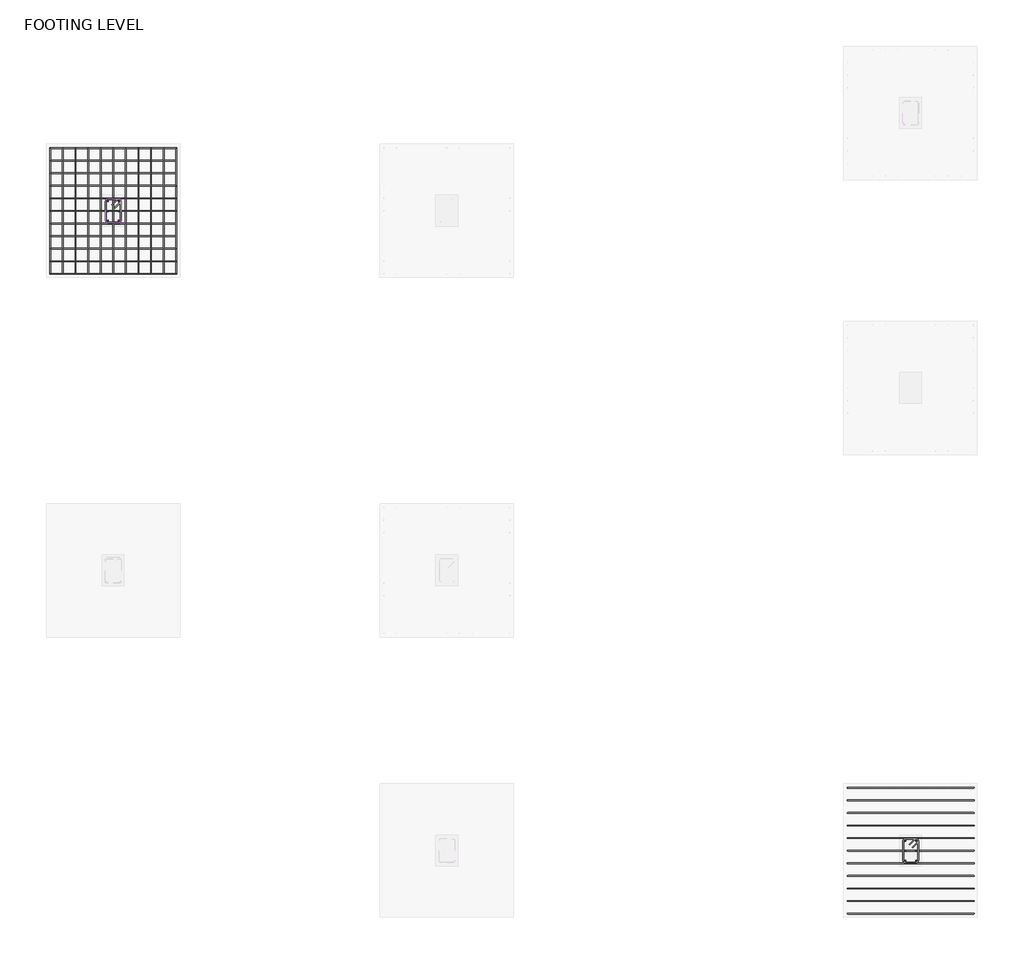
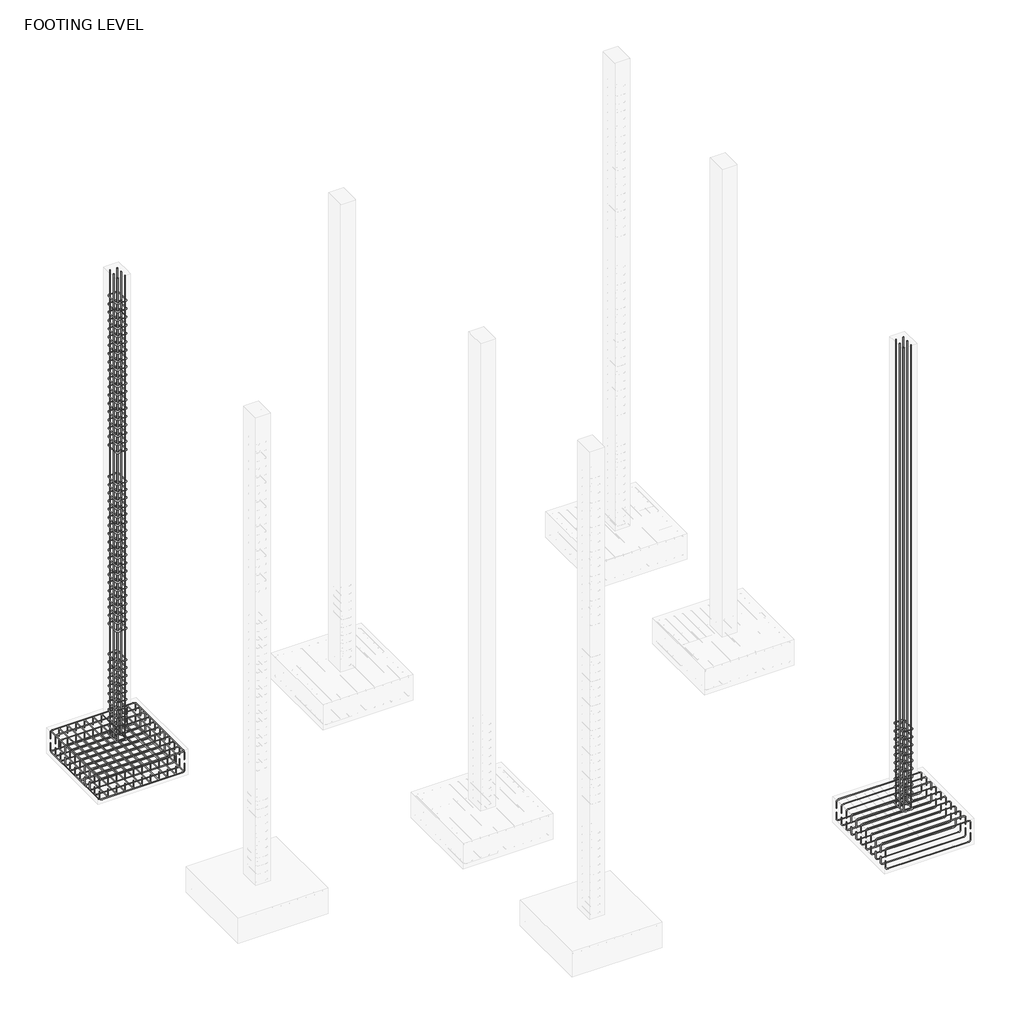
# One storey, part 4 of 9: 22 reinforcing bars.
"""IFC4 building model written with IfcOpenShell, lengths in millimetres."""

from ifc_helpers import new_model, si_unit, point, frame, origin, place, context, project, spatial, polyline, circle_curve, trimmed, segment, composite_curve, source, transform, mapped, element, save
from ifc_brep_helpers import swept_disk

model = new_model("IFC4")

# Units and contexts
model_context = context("Model", 3, world=origin())
ifc_project = project(units=[si_unit("LENGTHUNIT", "METRE", prefix="MILLI")], contexts=[model_context])

# Site, building, storey
site = spatial("IfcSite", under=ifc_project)
building = spatial("IfcBuilding", under=site)
storey = spatial("IfcBuildingStorey", under=building, Name="FOOTING LEVEL", Elevation=-1981.2)

# Reinforcing bars
placement = place(None, origin())
reinforcing_bar_shape = source(origin(), model_context, "Body", "SolidModel", [
    swept_disk(composite_curve([segment(polyline([(-3975.4566189, -3042.2841598, -2171.7), (-3975.4566189, -3042.2841598, -2057.4)]), True, "CONTINUOUS"), segment(trimmed(circle_curve(frame((-3942.1191189, -3042.2841598, -2057.4), z_axis=(0.0, 1.0, 0.0), x_axis=(-33.33750000000009, 0.0, 0.0)), 33.3375), [point((-3975.4566189, -3042.2841598, -2057.4))], [point((-3942.1191189, -3042.2841598, -2024.0625))], True, "CARTESIAN"), True, "CONTINUOUS"), segment(polyline([(-3942.1191189, -3042.2841598, -2024.0625), (-2570.5191189, -3042.2841598, -2024.0625)]), True, "CONTINUOUS"), segment(trimmed(circle_curve(frame((-2570.5191189, -3042.2841598, -2057.4), z_axis=(0.0, 1.0, 0.0), x_axis=(0.0, 0.0, 33.33750000000009)), 33.3375), [point((-2570.5191189, -3042.2841598, -2024.0625))], [point((-2537.1816189, -3042.2841598, -2057.4))], True, "CARTESIAN"), True, "CONTINUOUS"), segment(polyline([(-2537.1816189, -3042.2841598, -2057.4), (-2537.1816189, -3042.2841598, -2171.7)]), True, "CONTINUOUS")], self_intersect=False), 4.7625),
])
element("IfcReinforcingBar", 1, at=placement, inside=storey, context=model_context, shape_type="MappedRepresentation", body=[
    mapped(reinforcing_bar_shape, transform((0.0, 0.0, 0.0), x_axis=(1.0, 0.0, 0.0), y_axis=(0.0, 1.0, 0.0), z_axis=(0.0, 0.0, 1.0))),
    mapped(reinforcing_bar_shape, transform((0.0, -143.8275, 0.0), x_axis=(1.0, 0.0, 0.0), y_axis=(0.0, 1.0, 0.0), z_axis=(0.0, 0.0, 1.0))),
    mapped(reinforcing_bar_shape, transform((0.0, -287.655, 0.0), x_axis=(1.0, 0.0, 0.0), y_axis=(0.0, 1.0, 0.0), z_axis=(0.0, 0.0, 1.0))),
    mapped(reinforcing_bar_shape, transform((0.0, -431.4825, 0.0), x_axis=(1.0, 0.0, 0.0), y_axis=(0.0, 1.0, 0.0), z_axis=(0.0, 0.0, 1.0))),
    mapped(reinforcing_bar_shape, transform((0.0, -575.31, 0.0), x_axis=(1.0, 0.0, 0.0), y_axis=(0.0, 1.0, 0.0), z_axis=(0.0, 0.0, 1.0))),
    mapped(reinforcing_bar_shape, transform((0.0, -719.1375, 0.0), x_axis=(1.0, 0.0, 0.0), y_axis=(0.0, 1.0, 0.0), z_axis=(0.0, 0.0, 1.0))),
    mapped(reinforcing_bar_shape, transform((0.0, -862.965, 0.0), x_axis=(1.0, 0.0, 0.0), y_axis=(0.0, 1.0, 0.0), z_axis=(0.0, 0.0, 1.0))),
    mapped(reinforcing_bar_shape, transform((0.0, -1006.7925, 0.0), x_axis=(1.0, 0.0, 0.0), y_axis=(0.0, 1.0, 0.0), z_axis=(0.0, 0.0, 1.0))),
    mapped(reinforcing_bar_shape, transform((0.0, -1150.62, 0.0), x_axis=(1.0, 0.0, 0.0), y_axis=(0.0, 1.0, 0.0), z_axis=(0.0, 0.0, 1.0))),
    mapped(reinforcing_bar_shape, transform((0.0, -1294.4475, 0.0), x_axis=(1.0, 0.0, 0.0), y_axis=(0.0, 1.0, 0.0), z_axis=(0.0, 0.0, 1.0))),
    mapped(reinforcing_bar_shape, transform((0.0, -1438.275, 0.0), x_axis=(1.0, 0.0, 0.0), y_axis=(0.0, 1.0, 0.0), z_axis=(0.0, 0.0, 1.0))),
])
reinforcing_bar_2_shape = source(origin(), model_context, "Body", "SolidModel", [
    swept_disk(composite_curve([segment(polyline([(-3975.4566189, -4480.5591598, -2247.9), (-3975.4566189, -4480.5591598, -2362.2)]), True, "CONTINUOUS"), segment(trimmed(circle_curve(frame((-3942.1191189, -4480.5591598, -2362.2), z_axis=(0.0, -1.0, 0.0), x_axis=(-33.33750000000009, 0.0, 0.0)), 33.3375), [point((-3975.4566189, -4480.5591598, -2362.2))], [point((-3942.1191189, -4480.5591598, -2395.5375))], True, "CARTESIAN"), True, "CONTINUOUS"), segment(polyline([(-3942.1191189, -4480.5591598, -2395.5375), (-2570.5191189, -4480.5591598, -2395.5375)]), True, "CONTINUOUS"), segment(trimmed(circle_curve(frame((-2570.5191189, -4480.5591598, -2362.2), z_axis=(0.0, -1.0, 0.0), x_axis=(0.0, 0.0, -33.33750000000009)), 33.3375), [point((-2570.5191189, -4480.5591598, -2395.5375))], [point((-2537.1816189, -4480.5591598, -2362.2))], True, "CARTESIAN"), True, "CONTINUOUS"), segment(polyline([(-2537.1816189, -4480.5591598, -2362.2), (-2537.1816189, -4480.5591598, -2247.9)]), True, "CONTINUOUS")], self_intersect=False), 4.7625),
])
element("IfcReinforcingBar", 2, at=placement, inside=storey, context=model_context, shape_type="MappedRepresentation", body=[
    mapped(reinforcing_bar_2_shape, transform((0.0, 0.0, 0.0), x_axis=(1.0, 0.0, 0.0), y_axis=(0.0, 1.0, 0.0), z_axis=(0.0, 0.0, 1.0))),
    mapped(reinforcing_bar_2_shape, transform((0.0, 143.8275, 0.0), x_axis=(1.0, 0.0, 0.0), y_axis=(0.0, 1.0, 0.0), z_axis=(0.0, 0.0, 1.0))),
    mapped(reinforcing_bar_2_shape, transform((0.0, 287.655, 0.0), x_axis=(1.0, 0.0, 0.0), y_axis=(0.0, 1.0, 0.0), z_axis=(0.0, 0.0, 1.0))),
    mapped(reinforcing_bar_2_shape, transform((0.0, 431.4825, 0.0), x_axis=(1.0, 0.0, 0.0), y_axis=(0.0, 1.0, 0.0), z_axis=(0.0, 0.0, 1.0))),
    mapped(reinforcing_bar_2_shape, transform((0.0, 575.31, 0.0), x_axis=(1.0, 0.0, 0.0), y_axis=(0.0, 1.0, 0.0), z_axis=(0.0, 0.0, 1.0))),
    mapped(reinforcing_bar_2_shape, transform((0.0, 719.1375, 0.0), x_axis=(1.0, 0.0, 0.0), y_axis=(0.0, 1.0, 0.0), z_axis=(0.0, 0.0, 1.0))),
    mapped(reinforcing_bar_2_shape, transform((0.0, 862.965, 0.0), x_axis=(1.0, 0.0, 0.0), y_axis=(0.0, 1.0, 0.0), z_axis=(0.0, 0.0, 1.0))),
    mapped(reinforcing_bar_2_shape, transform((0.0, 1006.7925, 0.0), x_axis=(1.0, 0.0, 0.0), y_axis=(0.0, 1.0, 0.0), z_axis=(0.0, 0.0, 1.0))),
    mapped(reinforcing_bar_2_shape, transform((0.0, 1150.62, 0.0), x_axis=(1.0, 0.0, 0.0), y_axis=(0.0, 1.0, 0.0), z_axis=(0.0, 0.0, 1.0))),
    mapped(reinforcing_bar_2_shape, transform((0.0, 1294.4475, 0.0), x_axis=(1.0, 0.0, 0.0), y_axis=(0.0, 1.0, 0.0), z_axis=(0.0, 0.0, 1.0))),
    mapped(reinforcing_bar_2_shape, transform((0.0, 1438.275, 0.0), x_axis=(1.0, 0.0, 0.0), y_axis=(0.0, 1.0, 0.0), z_axis=(0.0, 0.0, 1.0))),
])
reinforcing_bar_3_shape = source(origin(), model_context, "Body", "SolidModel", [
    swept_disk(composite_curve([segment(polyline([(-11642.9458659, 4266.5658402, -2171.7), (-11642.9458659, 4266.5658402, -2057.4)]), True, "CONTINUOUS"), segment(trimmed(circle_curve(frame((-11642.9458659, 4233.2283402, -2057.4), z_axis=(1.0, 0.0, 0.0), x_axis=(0.0, 33.337499999999636, 0.0)), 33.3375), [point((-11642.9458659, 4266.5658402, -2057.4))], [point((-11642.9458659, 4233.2283402, -2024.0625))], True, "CARTESIAN"), True, "CONTINUOUS"), segment(polyline([(-11642.9458659, 4233.2283402, -2024.0625), (-11642.9458659, 2861.6283402, -2024.0625)]), True, "CONTINUOUS"), segment(trimmed(circle_curve(frame((-11642.9458659, 2861.6283402, -2057.4), z_axis=(1.0, 0.0, 0.0), x_axis=(0.0, 0.0, 33.33750000000009)), 33.3375), [point((-11642.9458659, 2861.6283402, -2024.0625))], [point((-11642.9458659, 2828.2908402, -2057.4))], True, "CARTESIAN"), True, "CONTINUOUS"), segment(polyline([(-11642.9458659, 2828.2908402, -2057.4), (-11642.9458659, 2828.2908402, -2171.7)]), True, "CONTINUOUS")], self_intersect=False), 4.7625),
])
element("IfcReinforcingBar", 3, at=placement, inside=storey, context=model_context, shape_type="MappedRepresentation", body=[
    mapped(reinforcing_bar_3_shape, transform((0.0, 0.0, 0.0), x_axis=(1.0, 0.0, 0.0), y_axis=(0.0, 1.0, 0.0), z_axis=(0.0, 0.0, 1.0))),
    mapped(reinforcing_bar_3_shape, transform((-143.8275, 0.0, 0.0), x_axis=(1.0, 0.0, 0.0), y_axis=(0.0, 1.0, 0.0), z_axis=(0.0, 0.0, 1.0))),
    mapped(reinforcing_bar_3_shape, transform((-287.655, 0.0, 0.0), x_axis=(1.0, 0.0, 0.0), y_axis=(0.0, 1.0, 0.0), z_axis=(0.0, 0.0, 1.0))),
    mapped(reinforcing_bar_3_shape, transform((-431.4825, 0.0, 0.0), x_axis=(1.0, 0.0, 0.0), y_axis=(0.0, 1.0, 0.0), z_axis=(0.0, 0.0, 1.0))),
    mapped(reinforcing_bar_3_shape, transform((-575.31, 0.0, 0.0), x_axis=(1.0, 0.0, 0.0), y_axis=(0.0, 1.0, 0.0), z_axis=(0.0, 0.0, 1.0))),
    mapped(reinforcing_bar_3_shape, transform((-719.1375, 0.0, 0.0), x_axis=(1.0, 0.0, 0.0), y_axis=(0.0, 1.0, 0.0), z_axis=(0.0, 0.0, 1.0))),
    mapped(reinforcing_bar_3_shape, transform((-862.965, 0.0, 0.0), x_axis=(1.0, 0.0, 0.0), y_axis=(0.0, 1.0, 0.0), z_axis=(0.0, 0.0, 1.0))),
    mapped(reinforcing_bar_3_shape, transform((-1006.7925, 0.0, 0.0), x_axis=(1.0, 0.0, 0.0), y_axis=(0.0, 1.0, 0.0), z_axis=(0.0, 0.0, 1.0))),
    mapped(reinforcing_bar_3_shape, transform((-1150.62, 0.0, 0.0), x_axis=(1.0, 0.0, 0.0), y_axis=(0.0, 1.0, 0.0), z_axis=(0.0, 0.0, 1.0))),
    mapped(reinforcing_bar_3_shape, transform((-1294.4475, 0.0, 0.0), x_axis=(1.0, 0.0, 0.0), y_axis=(0.0, 1.0, 0.0), z_axis=(0.0, 0.0, 1.0))),
    mapped(reinforcing_bar_3_shape, transform((-1438.275, 0.0, 0.0), x_axis=(1.0, 0.0, 0.0), y_axis=(0.0, 1.0, 0.0), z_axis=(0.0, 0.0, 1.0))),
])
reinforcing_bar_4_shape = source(origin(), model_context, "Body", "SolidModel", [
    swept_disk(composite_curve([segment(polyline([(-11642.9458659, 2828.2908402, -2247.9), (-11642.9458659, 2828.2908402, -2362.2)]), True, "CONTINUOUS"), segment(trimmed(circle_curve(frame((-11642.9458659, 2861.6283402, -2362.2), z_axis=(1.0, 0.0, 0.0), x_axis=(0.0, -33.33750000000009, 0.0)), 33.3375), [point((-11642.9458659, 2828.2908402, -2362.2))], [point((-11642.9458659, 2861.6283402, -2395.5375))], True, "CARTESIAN"), True, "CONTINUOUS"), segment(polyline([(-11642.9458659, 2861.6283402, -2395.5375), (-11642.9458659, 4233.2283402, -2395.5375)]), True, "CONTINUOUS"), segment(trimmed(circle_curve(frame((-11642.9458659, 4233.2283402, -2362.2), z_axis=(1.0, 0.0, 0.0), x_axis=(0.0, 0.0, -33.33750000000009)), 33.3375), [point((-11642.9458659, 4233.2283402, -2395.5375))], [point((-11642.9458659, 4266.5658402, -2362.2))], True, "CARTESIAN"), True, "CONTINUOUS"), segment(polyline([(-11642.9458659, 4266.5658402, -2362.2), (-11642.9458659, 4266.5658402, -2247.9)]), True, "CONTINUOUS")], self_intersect=False), 4.7625),
])
element("IfcReinforcingBar", 4, at=placement, inside=storey, context=model_context, shape_type="MappedRepresentation", body=[
    mapped(reinforcing_bar_4_shape, transform((0.0, 0.0, 0.0), x_axis=(1.0, 0.0, 0.0), y_axis=(0.0, 1.0, 0.0), z_axis=(0.0, 0.0, 1.0))),
    mapped(reinforcing_bar_4_shape, transform((-143.8275, 0.0, 0.0), x_axis=(1.0, 0.0, 0.0), y_axis=(0.0, 1.0, 0.0), z_axis=(0.0, 0.0, 1.0))),
    mapped(reinforcing_bar_4_shape, transform((-287.655, 0.0, 0.0), x_axis=(1.0, 0.0, 0.0), y_axis=(0.0, 1.0, 0.0), z_axis=(0.0, 0.0, 1.0))),
    mapped(reinforcing_bar_4_shape, transform((-431.4825, 0.0, 0.0), x_axis=(1.0, 0.0, 0.0), y_axis=(0.0, 1.0, 0.0), z_axis=(0.0, 0.0, 1.0))),
    mapped(reinforcing_bar_4_shape, transform((-575.31, 0.0, 0.0), x_axis=(1.0, 0.0, 0.0), y_axis=(0.0, 1.0, 0.0), z_axis=(0.0, 0.0, 1.0))),
    mapped(reinforcing_bar_4_shape, transform((-719.1375, 0.0, 0.0), x_axis=(1.0, 0.0, 0.0), y_axis=(0.0, 1.0, 0.0), z_axis=(0.0, 0.0, 1.0))),
    mapped(reinforcing_bar_4_shape, transform((-862.965, 0.0, 0.0), x_axis=(1.0, 0.0, 0.0), y_axis=(0.0, 1.0, 0.0), z_axis=(0.0, 0.0, 1.0))),
    mapped(reinforcing_bar_4_shape, transform((-1006.7925, 0.0, 0.0), x_axis=(1.0, 0.0, 0.0), y_axis=(0.0, 1.0, 0.0), z_axis=(0.0, 0.0, 1.0))),
    mapped(reinforcing_bar_4_shape, transform((-1150.62, 0.0, 0.0), x_axis=(1.0, 0.0, 0.0), y_axis=(0.0, 1.0, 0.0), z_axis=(0.0, 0.0, 1.0))),
    mapped(reinforcing_bar_4_shape, transform((-1294.4475, 0.0, 0.0), x_axis=(1.0, 0.0, 0.0), y_axis=(0.0, 1.0, 0.0), z_axis=(0.0, 0.0, 1.0))),
    mapped(reinforcing_bar_4_shape, transform((-1438.275, 0.0, 0.0), x_axis=(1.0, 0.0, 0.0), y_axis=(0.0, 1.0, 0.0), z_axis=(0.0, 0.0, 1.0))),
])
reinforcing_bar_5_shape = source(origin(), model_context, "Body", "SolidModel", [
    swept_disk(composite_curve([segment(polyline([(-13081.2208659, 4266.5658402, -2171.7), (-13081.2208659, 4266.5658402, -2057.4)]), True, "CONTINUOUS"), segment(trimmed(circle_curve(frame((-13047.8833659, 4266.5658402, -2057.4), z_axis=(0.0, 1.0, 0.0), x_axis=(-33.337500000001455, 0.0, 0.0)), 33.3375), [point((-13081.2208659, 4266.5658402, -2057.4))], [point((-13047.8833659, 4266.5658402, -2024.0625))], True, "CARTESIAN"), True, "CONTINUOUS"), segment(polyline([(-13047.8833659, 4266.5658402, -2024.0625), (-11676.2833659, 4266.5658402, -2024.0625)]), True, "CONTINUOUS"), segment(trimmed(circle_curve(frame((-11676.2833659, 4266.5658402, -2057.4), z_axis=(0.0, 1.0, 0.0), x_axis=(0.0, 0.0, 33.33750000000009)), 33.3375), [point((-11676.2833659, 4266.5658402, -2024.0625))], [point((-11642.9458659, 4266.5658402, -2057.4))], True, "CARTESIAN"), True, "CONTINUOUS"), segment(polyline([(-11642.9458659, 4266.5658402, -2057.4), (-11642.9458659, 4266.5658402, -2171.7)]), True, "CONTINUOUS")], self_intersect=False), 4.7625),
])
element("IfcReinforcingBar", 5, at=placement, inside=storey, context=model_context, shape_type="MappedRepresentation", body=[
    mapped(reinforcing_bar_5_shape, transform((0.0, 0.0, 0.0), x_axis=(1.0, 0.0, 0.0), y_axis=(0.0, 1.0, 0.0), z_axis=(0.0, 0.0, 1.0))),
    mapped(reinforcing_bar_5_shape, transform((0.0, -143.8275, 0.0), x_axis=(1.0, 0.0, 0.0), y_axis=(0.0, 1.0, 0.0), z_axis=(0.0, 0.0, 1.0))),
    mapped(reinforcing_bar_5_shape, transform((0.0, -287.655, 0.0), x_axis=(1.0, 0.0, 0.0), y_axis=(0.0, 1.0, 0.0), z_axis=(0.0, 0.0, 1.0))),
    mapped(reinforcing_bar_5_shape, transform((0.0, -431.4825, 0.0), x_axis=(1.0, 0.0, 0.0), y_axis=(0.0, 1.0, 0.0), z_axis=(0.0, 0.0, 1.0))),
    mapped(reinforcing_bar_5_shape, transform((0.0, -575.31, 0.0), x_axis=(1.0, 0.0, 0.0), y_axis=(0.0, 1.0, 0.0), z_axis=(0.0, 0.0, 1.0))),
    mapped(reinforcing_bar_5_shape, transform((0.0, -719.1375, 0.0), x_axis=(1.0, 0.0, 0.0), y_axis=(0.0, 1.0, 0.0), z_axis=(0.0, 0.0, 1.0))),
    mapped(reinforcing_bar_5_shape, transform((0.0, -862.965, 0.0), x_axis=(1.0, 0.0, 0.0), y_axis=(0.0, 1.0, 0.0), z_axis=(0.0, 0.0, 1.0))),
    mapped(reinforcing_bar_5_shape, transform((0.0, -1006.7925, 0.0), x_axis=(1.0, 0.0, 0.0), y_axis=(0.0, 1.0, 0.0), z_axis=(0.0, 0.0, 1.0))),
    mapped(reinforcing_bar_5_shape, transform((0.0, -1150.62, 0.0), x_axis=(1.0, 0.0, 0.0), y_axis=(0.0, 1.0, 0.0), z_axis=(0.0, 0.0, 1.0))),
    mapped(reinforcing_bar_5_shape, transform((0.0, -1294.4475, 0.0), x_axis=(1.0, 0.0, 0.0), y_axis=(0.0, 1.0, 0.0), z_axis=(0.0, 0.0, 1.0))),
    mapped(reinforcing_bar_5_shape, transform((0.0, -1438.275, 0.0), x_axis=(1.0, 0.0, 0.0), y_axis=(0.0, 1.0, 0.0), z_axis=(0.0, 0.0, 1.0))),
])
reinforcing_bar_6_shape = source(origin(), model_context, "Body", "SolidModel", [
    swept_disk(composite_curve([segment(polyline([(-13081.2208659, 2828.2908402, -2247.9), (-13081.2208659, 2828.2908402, -2362.2)]), True, "CONTINUOUS"), segment(trimmed(circle_curve(frame((-13047.8833659, 2828.2908402, -2362.2), z_axis=(0.0, -1.0, 0.0), x_axis=(-33.337500000001455, 0.0, 0.0)), 33.3375), [point((-13081.2208659, 2828.2908402, -2362.2))], [point((-13047.8833659, 2828.2908402, -2395.5375))], True, "CARTESIAN"), True, "CONTINUOUS"), segment(polyline([(-13047.8833659, 2828.2908402, -2395.5375), (-11676.2833659, 2828.2908402, -2395.5375)]), True, "CONTINUOUS"), segment(trimmed(circle_curve(frame((-11676.2833659, 2828.2908402, -2362.2), z_axis=(0.0, -1.0, 0.0), x_axis=(0.0, 0.0, -33.33750000000009)), 33.3375), [point((-11676.2833659, 2828.2908402, -2395.5375))], [point((-11642.9458659, 2828.2908402, -2362.2))], True, "CARTESIAN"), True, "CONTINUOUS"), segment(polyline([(-11642.9458659, 2828.2908402, -2362.2), (-11642.9458659, 2828.2908402, -2247.9)]), True, "CONTINUOUS")], self_intersect=False), 4.7625),
])
element("IfcReinforcingBar", 6, at=placement, inside=storey, context=model_context, shape_type="MappedRepresentation", body=[
    mapped(reinforcing_bar_6_shape, transform((0.0, 0.0, 0.0), x_axis=(1.0, 0.0, 0.0), y_axis=(0.0, 1.0, 0.0), z_axis=(0.0, 0.0, 1.0))),
    mapped(reinforcing_bar_6_shape, transform((0.0, 143.8275, 0.0), x_axis=(1.0, 0.0, 0.0), y_axis=(0.0, 1.0, 0.0), z_axis=(0.0, 0.0, 1.0))),
    mapped(reinforcing_bar_6_shape, transform((0.0, 287.655, 0.0), x_axis=(1.0, 0.0, 0.0), y_axis=(0.0, 1.0, 0.0), z_axis=(0.0, 0.0, 1.0))),
    mapped(reinforcing_bar_6_shape, transform((0.0, 431.4825, 0.0), x_axis=(1.0, 0.0, 0.0), y_axis=(0.0, 1.0, 0.0), z_axis=(0.0, 0.0, 1.0))),
    mapped(reinforcing_bar_6_shape, transform((0.0, 575.31, 0.0), x_axis=(1.0, 0.0, 0.0), y_axis=(0.0, 1.0, 0.0), z_axis=(0.0, 0.0, 1.0))),
    mapped(reinforcing_bar_6_shape, transform((0.0, 719.1375, 0.0), x_axis=(1.0, 0.0, 0.0), y_axis=(0.0, 1.0, 0.0), z_axis=(0.0, 0.0, 1.0))),
    mapped(reinforcing_bar_6_shape, transform((0.0, 862.965, 0.0), x_axis=(1.0, 0.0, 0.0), y_axis=(0.0, 1.0, 0.0), z_axis=(0.0, 0.0, 1.0))),
    mapped(reinforcing_bar_6_shape, transform((0.0, 1006.7925, 0.0), x_axis=(1.0, 0.0, 0.0), y_axis=(0.0, 1.0, 0.0), z_axis=(0.0, 0.0, 1.0))),
    mapped(reinforcing_bar_6_shape, transform((0.0, 1150.62, 0.0), x_axis=(1.0, 0.0, 0.0), y_axis=(0.0, 1.0, 0.0), z_axis=(0.0, 0.0, 1.0))),
    mapped(reinforcing_bar_6_shape, transform((0.0, 1294.4475, 0.0), x_axis=(1.0, 0.0, 0.0), y_axis=(0.0, 1.0, 0.0), z_axis=(0.0, 0.0, 1.0))),
    mapped(reinforcing_bar_6_shape, transform((0.0, 1438.275, 0.0), x_axis=(1.0, 0.0, 0.0), y_axis=(0.0, 1.0, 0.0), z_axis=(0.0, 0.0, 1.0))),
])
reinforcing_bar_7_shape = source(origin(), model_context, "Body", "SolidModel", [
    swept_disk(composite_curve([segment(polyline([(-12341.7845827, 3584.8511629, -1938.3375), (-12284.9203857, 3641.71536, -1938.3375)]), True, "CONTINUOUS"), segment(trimmed(circle_curve(frame((-12301.7583659, 3658.5533402, -1938.3375), z_axis=(0.0, 0.0, 1.0), x_axis=(16.837980199999947, -16.837980199999947, 0.0)), 23.8125), [point((-12284.9203857, 3641.71536, -1938.3375))], [point((-12301.7583659, 3682.3658402, -1938.3375))], True, "CARTESIAN"), True, "CONTINUOUS"), segment(polyline([(-12301.7583659, 3682.3658402, -1938.3375), (-12422.4083659, 3682.3658402, -1938.3375)]), True, "CONTINUOUS"), segment(trimmed(circle_curve(frame((-12422.4083659, 3658.5533402, -1938.3375), z_axis=(0.0, 0.0, 1.0), x_axis=(0.0, 23.8125, 0.0)), 23.8125), [point((-12422.4083659, 3682.3658402, -1938.3375))], [point((-12446.2208659, 3658.5533402, -1938.3375))], True, "CARTESIAN"), True, "CONTINUOUS"), segment(polyline([(-12446.2208659, 3658.5533402, -1938.3375), (-12446.2208659, 3436.3033402, -1938.3375)]), True, "CONTINUOUS"), segment(trimmed(circle_curve(frame((-12422.4464219, 3436.3033402, -1939.6832232), z_axis=(0.056513312022656255, 0.0, 0.9984018457335854), x_axis=(-23.774444000000585, 0.0, 1.3457231999998385)), 23.8125), [point((-12446.2208659, 3436.3033402, -1938.3375))], [point((-12422.4464219, 3412.4908402, -1939.6832232))], True, "CARTESIAN"), True, "CONTINUOUS"), segment(polyline([(-12422.4464219, 3412.4908402, -1939.6832232), (-12301.7203098, 3412.4908402, -1946.5167768)]), True, "CONTINUOUS"), segment(trimmed(circle_curve(frame((-12301.7203098, 3436.3033402, -1946.5167768), z_axis=(0.056513312022656255, 0.0, 0.9984018457335854), x_axis=(0.0, -23.8125, 0.0)), 23.8125), [point((-12301.7203098, 3412.4908402, -1946.5167768))], [point((-12277.9458659, 3436.3033402, -1947.8625))], True, "CARTESIAN"), True, "CONTINUOUS"), segment(polyline([(-12277.9458659, 3436.3033402, -1947.8625), (-12277.9458659, 3658.5533402, -1947.8625)]), True, "CONTINUOUS"), segment(trimmed(circle_curve(frame((-12301.7583659, 3658.5533402, -1947.8625), z_axis=(0.0, 0.0, 1.0), x_axis=(23.8125, 0.0, 0.0)), 23.8125), [point((-12277.9458659, 3658.5533402, -1947.8625))], [point((-12318.5963461, 3675.3913204, -1947.8625))], True, "CARTESIAN"), True, "CONTINUOUS"), segment(polyline([(-12318.5963461, 3675.3913204, -1947.8625), (-12375.4605432, 3618.5271233, -1947.8625)]), True, "CONTINUOUS")], self_intersect=False), 4.7625),
])
element("IfcReinforcingBar", 7, at=placement, inside=storey, context=model_context, shape_type="MappedRepresentation", body=[
    mapped(reinforcing_bar_7_shape, transform((0.0, 0.0, 0.0), x_axis=(1.0, 0.0, 0.0), y_axis=(0.0, 1.0, 0.0), z_axis=(0.0, 0.0, 1.0))),
    mapped(reinforcing_bar_7_shape, transform((0.0, 0.0, 142.5866456), x_axis=(1.0, 0.0, 0.0), y_axis=(0.0, 1.0, 0.0), z_axis=(0.0, 0.0, 1.0))),
    mapped(reinforcing_bar_7_shape, transform((0.0, 0.0, 285.1732912), x_axis=(1.0, 0.0, 0.0), y_axis=(0.0, 1.0, 0.0), z_axis=(0.0, 0.0, 1.0))),
    mapped(reinforcing_bar_7_shape, transform((0.0, 0.0, 427.7599369), x_axis=(1.0, 0.0, 0.0), y_axis=(0.0, 1.0, 0.0), z_axis=(0.0, 0.0, 1.0))),
    mapped(reinforcing_bar_7_shape, transform((0.0, 0.0, 570.3465825), x_axis=(1.0, 0.0, 0.0), y_axis=(0.0, 1.0, 0.0), z_axis=(0.0, 0.0, 1.0))),
    mapped(reinforcing_bar_7_shape, transform((0.0, 0.0, 712.9332281), x_axis=(1.0, 0.0, 0.0), y_axis=(0.0, 1.0, 0.0), z_axis=(0.0, 0.0, 1.0))),
    mapped(reinforcing_bar_7_shape, transform((0.0, 0.0, 855.5198737), x_axis=(1.0, 0.0, 0.0), y_axis=(0.0, 1.0, 0.0), z_axis=(0.0, 0.0, 1.0))),
    mapped(reinforcing_bar_7_shape, transform((0.0, 0.0, 998.1065193), x_axis=(1.0, 0.0, 0.0), y_axis=(0.0, 1.0, 0.0), z_axis=(0.0, 0.0, 1.0))),
    mapped(reinforcing_bar_7_shape, transform((0.0, 0.0, 1140.6931649), x_axis=(1.0, 0.0, 0.0), y_axis=(0.0, 1.0, 0.0), z_axis=(0.0, 0.0, 1.0))),
    mapped(reinforcing_bar_7_shape, transform((0.0, 0.0, 1283.2798106), x_axis=(1.0, 0.0, 0.0), y_axis=(0.0, 1.0, 0.0), z_axis=(0.0, 0.0, 1.0))),
    mapped(reinforcing_bar_7_shape, transform((0.0, 0.0, 1425.8664562), x_axis=(1.0, 0.0, 0.0), y_axis=(0.0, 1.0, 0.0), z_axis=(0.0, 0.0, 1.0))),
])
element("IfcReinforcingBar", 8, at=placement, inside=storey, context=model_context, shape_type="SolidModel", body=[
    swept_disk(composite_curve([segment(polyline([(-12300.2784581, 3433.9470011, -1943.1), (-12300.2784581, 3433.9470011, 6362.7)]), True, "CONTINUOUS")], self_intersect=False), 6.35),
])
element("IfcReinforcingBar", 9, at=placement, inside=storey, context=model_context, shape_type="SolidModel", body=[
    swept_disk(composite_curve([segment(polyline([(-12423.8882737, 3433.9470011, -1943.1), (-12423.8882737, 3433.9470011, 6362.7)]), True, "CONTINUOUS")], self_intersect=False), 6.35),
])
element("IfcReinforcingBar", 10, at=placement, inside=storey, context=model_context, shape_type="SolidModel", body=[
    swept_disk(composite_curve([segment(polyline([(-12300.2784581, 3660.9096793, -1943.1), (-12300.2784581, 3660.9096793, 6362.7)]), True, "CONTINUOUS")], self_intersect=False), 6.35),
])
element("IfcReinforcingBar", 11, at=placement, inside=storey, context=model_context, shape_type="SolidModel", body=[
    swept_disk(composite_curve([segment(polyline([(-12423.8882737, 3660.9096793, -1943.1), (-12423.8882737, 3660.9096793, 6362.7)]), True, "CONTINUOUS")], self_intersect=False), 6.35),
])
element("IfcReinforcingBar", 12, at=placement, inside=storey, context=model_context, shape_type="SolidModel", body=[
    swept_disk(composite_curve([segment(polyline([(-12300.2784581, 3546.6096793, -1943.1), (-12300.2784581, 3546.6096793, 6362.7)]), True, "CONTINUOUS")], self_intersect=False), 6.35),
])
element("IfcReinforcingBar", 13, at=placement, inside=storey, context=model_context, shape_type="SolidModel", body=[
    swept_disk(composite_curve([segment(polyline([(-12423.8882737, 3546.6096793, -1943.1), (-12423.8882737, 3546.6096793, 6362.7)]), True, "CONTINUOUS")], self_intersect=False), 6.35),
])
reinforcing_bar_8_shape = source(origin(), model_context, "Body", "SolidModel", [
    swept_disk(composite_curve([segment(polyline([(-3236.0203358, -3723.9988371, -1938.3375), (-3179.1561387, -3667.13464, -1938.3375)]), True, "CONTINUOUS"), segment(trimmed(circle_curve(frame((-3195.9941189, -3650.2966598, -1938.3375), z_axis=(0.0, 0.0, 1.0), x_axis=(16.837980199999947, -16.837980200000402, 0.0)), 23.8125), [point((-3179.1561387, -3667.13464, -1938.3375))], [point((-3195.9941189, -3626.4841598, -1938.3375))], True, "CARTESIAN"), True, "CONTINUOUS"), segment(polyline([(-3195.9941189, -3626.4841598, -1938.3375), (-3316.6441189, -3626.4841598, -1938.3375)]), True, "CONTINUOUS"), segment(trimmed(circle_curve(frame((-3316.6441189, -3650.2966598, -1938.3375), z_axis=(0.0, 0.0, 1.0), x_axis=(0.0, 23.8125, 0.0)), 23.8125), [point((-3316.6441189, -3626.4841598, -1938.3375))], [point((-3340.4566189, -3650.2966598, -1938.3375))], True, "CARTESIAN"), True, "CONTINUOUS"), segment(polyline([(-3340.4566189, -3650.2966598, -1938.3375), (-3340.4566189, -3872.5466598, -1938.3375)]), True, "CONTINUOUS"), segment(trimmed(circle_curve(frame((-3316.682175, -3872.5466598, -1939.6832232), z_axis=(0.056513312022656255, 0.0, 0.9984018457335854), x_axis=(-23.77444390000028, 0.0, 1.3457231999998385)), 23.8125), [point((-3340.4566189, -3872.5466598, -1938.3375))], [point((-3316.682175, -3896.3591598, -1939.6832232))], True, "CARTESIAN"), True, "CONTINUOUS"), segment(polyline([(-3316.682175, -3896.3591598, -1939.6832232), (-3195.9560629, -3896.3591598, -1946.5167768)]), True, "CONTINUOUS"), segment(trimmed(circle_curve(frame((-3195.9560629, -3872.5466598, -1946.5167768), z_axis=(0.056513312022656255, 0.0, 0.9984018457335854), x_axis=(0.0, -23.8125, 0.0)), 23.8125), [point((-3195.9560629, -3896.3591598, -1946.5167768))], [point((-3172.1816189, -3872.5466598, -1947.8625))], True, "CARTESIAN"), True, "CONTINUOUS"), segment(polyline([(-3172.1816189, -3872.5466598, -1947.8625), (-3172.1816189, -3650.2966598, -1947.8625)]), True, "CONTINUOUS"), segment(trimmed(circle_curve(frame((-3195.9941189, -3650.2966598, -1947.8625), z_axis=(0.0, 0.0, 1.0), x_axis=(23.8125, 0.0, 0.0)), 23.8125), [point((-3172.1816189, -3650.2966598, -1947.8625))], [point((-3212.8320991, -3633.4586796, -1947.8625))], True, "CARTESIAN"), True, "CONTINUOUS"), segment(polyline([(-3212.8320991, -3633.4586796, -1947.8625), (-3269.6962962, -3690.3228767, -1947.8625)]), True, "CONTINUOUS")], self_intersect=False), 4.7625),
])
element("IfcReinforcingBar", 14, at=placement, inside=storey, context=model_context, shape_type="MappedRepresentation", body=[
    mapped(reinforcing_bar_8_shape, transform((0.0, 0.0, 0.0), x_axis=(1.0, 0.0, 0.0), y_axis=(0.0, 1.0, 0.0), z_axis=(0.0, 0.0, 1.0))),
    mapped(reinforcing_bar_8_shape, transform((0.0, 0.0, 142.9363281), x_axis=(1.0, 0.0, 0.0), y_axis=(0.0, 1.0, 0.0), z_axis=(0.0, 0.0, 1.0))),
    mapped(reinforcing_bar_8_shape, transform((0.0, 0.0, 285.8726562), x_axis=(1.0, 0.0, 0.0), y_axis=(0.0, 1.0, 0.0), z_axis=(0.0, 0.0, 1.0))),
    mapped(reinforcing_bar_8_shape, transform((0.0, 0.0, 428.8089844), x_axis=(1.0, 0.0, 0.0), y_axis=(0.0, 1.0, 0.0), z_axis=(0.0, 0.0, 1.0))),
    mapped(reinforcing_bar_8_shape, transform((0.0, 0.0, 571.7453125), x_axis=(1.0, 0.0, 0.0), y_axis=(0.0, 1.0, 0.0), z_axis=(0.0, 0.0, 1.0))),
    mapped(reinforcing_bar_8_shape, transform((0.0, 0.0, 714.6816406), x_axis=(1.0, 0.0, 0.0), y_axis=(0.0, 1.0, 0.0), z_axis=(0.0, 0.0, 1.0))),
    mapped(reinforcing_bar_8_shape, transform((0.0, 0.0, 857.6179687), x_axis=(1.0, 0.0, 0.0), y_axis=(0.0, 1.0, 0.0), z_axis=(0.0, 0.0, 1.0))),
    mapped(reinforcing_bar_8_shape, transform((0.0, 0.0, 1000.5542969), x_axis=(1.0, 0.0, 0.0), y_axis=(0.0, 1.0, 0.0), z_axis=(0.0, 0.0, 1.0))),
    mapped(reinforcing_bar_8_shape, transform((0.0, 0.0, 1143.490625), x_axis=(1.0, 0.0, 0.0), y_axis=(0.0, 1.0, 0.0), z_axis=(0.0, 0.0, 1.0))),
    mapped(reinforcing_bar_8_shape, transform((0.0, 0.0, 1286.4269531), x_axis=(1.0, 0.0, 0.0), y_axis=(0.0, 1.0, 0.0), z_axis=(0.0, 0.0, 1.0))),
    mapped(reinforcing_bar_8_shape, transform((0.0, 0.0, 1429.3632812), x_axis=(1.0, 0.0, 0.0), y_axis=(0.0, 1.0, 0.0), z_axis=(0.0, 0.0, 1.0))),
])
element("IfcReinforcingBar", 15, at=placement, inside=storey, context=model_context, shape_type="SolidModel", body=[
    swept_disk(composite_curve([segment(polyline([(-3194.5142111, -3874.9029989, -1943.1), (-3194.5142111, -3874.9029989, 6362.7)]), True, "CONTINUOUS")], self_intersect=False), 6.35),
])
element("IfcReinforcingBar", 16, at=placement, inside=storey, context=model_context, shape_type="SolidModel", body=[
    swept_disk(composite_curve([segment(polyline([(-3318.1240267, -3874.9029989, -1943.1), (-3318.1240267, -3874.9029989, 6362.7)]), True, "CONTINUOUS")], self_intersect=False), 6.35),
])
element("IfcReinforcingBar", 17, at=placement, inside=storey, context=model_context, shape_type="SolidModel", body=[
    swept_disk(composite_curve([segment(polyline([(-3194.5142111, -3647.9403207, -1943.1), (-3194.5142111, -3647.9403207, 6362.7)]), True, "CONTINUOUS")], self_intersect=False), 6.35),
])
element("IfcReinforcingBar", 18, at=placement, inside=storey, context=model_context, shape_type="SolidModel", body=[
    swept_disk(composite_curve([segment(polyline([(-3318.1240267, -3647.9403207, -1943.1), (-3318.1240267, -3647.9403207, 6362.7)]), True, "CONTINUOUS")], self_intersect=False), 6.35),
])
element("IfcReinforcingBar", 19, at=placement, inside=storey, context=model_context, shape_type="SolidModel", body=[
    swept_disk(composite_curve([segment(polyline([(-3194.5142111, -3762.2403207, -1943.1), (-3194.5142111, -3762.2403207, 6362.7)]), True, "CONTINUOUS")], self_intersect=False), 6.35),
])
element("IfcReinforcingBar", 20, at=placement, inside=storey, context=model_context, shape_type="SolidModel", body=[
    swept_disk(composite_curve([segment(polyline([(-3318.1240267, -3762.2403207, -1943.1), (-3318.1240267, -3762.2403207, 6362.7)]), True, "CONTINUOUS")], self_intersect=False), 6.35),
])
reinforcing_bar_9_shape = source(origin(), model_context, "Body", "SolidModel", [
    swept_disk(composite_curve([segment(polyline([(-12382.3821491, 3510.0055175, 42.8625), (-12439.2463461, 3453.1413204, 42.8625)]), True, "CONTINUOUS"), segment(trimmed(circle_curve(frame((-12422.4083659, 3436.3033402, 42.8625), z_axis=(0.0, 0.0, 1.0), x_axis=(-16.837980199999947, 16.837980199999947, 0.0)), 23.8125), [point((-12439.2463461, 3453.1413204, 42.8625))], [point((-12422.4083659, 3412.4908402, 42.8625))], True, "CARTESIAN"), True, "CONTINUOUS"), segment(polyline([(-12422.4083659, 3412.4908402, 42.8625), (-12301.7583659, 3412.4908402, 42.8625)]), True, "CONTINUOUS"), segment(trimmed(circle_curve(frame((-12301.7583659, 3436.3033402, 42.8625), z_axis=(0.0, 0.0, 1.0), x_axis=(0.0, -23.8125, 0.0)), 23.8125), [point((-12301.7583659, 3412.4908402, 42.8625))], [point((-12277.9458659, 3436.3033402, 42.8625))], True, "CARTESIAN"), True, "CONTINUOUS"), segment(polyline([(-12277.9458659, 3436.3033402, 42.8625), (-12277.9458659, 3658.5533402, 42.8625)]), True, "CONTINUOUS"), segment(trimmed(circle_curve(frame((-12301.7203098, 3658.5533402, 41.5167768), z_axis=(-0.056513312022656255, 0.0, 0.9984018457335854), x_axis=(23.774443900001643, 0.0, 1.3457231999999948)), 23.8125), [point((-12277.9458659, 3658.5533402, 42.8625))], [point((-12301.7203098, 3682.3658402, 41.5167768))], True, "CARTESIAN"), True, "CONTINUOUS"), segment(polyline([(-12301.7203098, 3682.3658402, 41.5167768), (-12422.4464219, 3682.3658402, 34.6832232)]), True, "CONTINUOUS"), segment(trimmed(circle_curve(frame((-12422.4464219, 3658.5533402, 34.6832232), z_axis=(-0.056513312022656255, 0.0, 0.9984018457335854), x_axis=(0.0, 23.8125, 0.0)), 23.8125), [point((-12422.4464219, 3682.3658402, 34.6832232))], [point((-12446.2208659, 3658.5533402, 33.3375))], True, "CARTESIAN"), True, "CONTINUOUS"), segment(polyline([(-12446.2208659, 3658.5533402, 33.3375), (-12446.2208659, 3436.3033402, 33.3375)]), True, "CONTINUOUS"), segment(trimmed(circle_curve(frame((-12422.4083659, 3436.3033402, 33.3375), z_axis=(0.0, 0.0, 1.0), x_axis=(-23.8125, 0.0, 0.0)), 23.8125), [point((-12446.2208659, 3436.3033402, 33.3375))], [point((-12405.5703857, 3419.46536, 33.3375))], True, "CARTESIAN"), True, "CONTINUOUS"), segment(polyline([(-12405.5703857, 3419.46536, 33.3375), (-12348.7061886, 3476.329557, 33.3375)]), True, "CONTINUOUS")], self_intersect=False), 4.7625),
])
element("IfcReinforcingBar", 21, at=placement, inside=storey, context=model_context, shape_type="MappedRepresentation", body=[
    mapped(reinforcing_bar_9_shape, transform((0.0, 0.0, 0.0), x_axis=(1.0, 0.0, 0.0), y_axis=(0.0, 1.0, 0.0), z_axis=(0.0, 0.0, 1.0))),
    mapped(reinforcing_bar_9_shape, transform((0.0, 0.0, 146.2204368), x_axis=(1.0, 0.0, 0.0), y_axis=(0.0, 1.0, 0.0), z_axis=(0.0, 0.0, 1.0))),
    mapped(reinforcing_bar_9_shape, transform((0.0, 0.0, 292.4408736), x_axis=(1.0, 0.0, 0.0), y_axis=(0.0, 1.0, 0.0), z_axis=(0.0, 0.0, 1.0))),
    mapped(reinforcing_bar_9_shape, transform((0.0, 0.0, 438.6613104), x_axis=(1.0, 0.0, 0.0), y_axis=(0.0, 1.0, 0.0), z_axis=(0.0, 0.0, 1.0))),
    mapped(reinforcing_bar_9_shape, transform((0.0, 0.0, 584.8817472), x_axis=(1.0, 0.0, 0.0), y_axis=(0.0, 1.0, 0.0), z_axis=(0.0, 0.0, 1.0))),
    mapped(reinforcing_bar_9_shape, transform((0.0, 0.0, 731.102184), x_axis=(1.0, 0.0, 0.0), y_axis=(0.0, 1.0, 0.0), z_axis=(0.0, 0.0, 1.0))),
    mapped(reinforcing_bar_9_shape, transform((0.0, 0.0, 877.3226208), x_axis=(1.0, 0.0, 0.0), y_axis=(0.0, 1.0, 0.0), z_axis=(0.0, 0.0, 1.0))),
    mapped(reinforcing_bar_9_shape, transform((0.0, 0.0, 1023.5430576), x_axis=(1.0, 0.0, 0.0), y_axis=(0.0, 1.0, 0.0), z_axis=(0.0, 0.0, 1.0))),
    mapped(reinforcing_bar_9_shape, transform((0.0, 0.0, 1169.7634944), x_axis=(1.0, 0.0, 0.0), y_axis=(0.0, 1.0, 0.0), z_axis=(0.0, 0.0, 1.0))),
    mapped(reinforcing_bar_9_shape, transform((0.0, 0.0, 1315.9839312), x_axis=(1.0, 0.0, 0.0), y_axis=(0.0, 1.0, 0.0), z_axis=(0.0, 0.0, 1.0))),
    mapped(reinforcing_bar_9_shape, transform((0.0, 0.0, 1462.2043681), x_axis=(1.0, 0.0, 0.0), y_axis=(0.0, 1.0, 0.0), z_axis=(0.0, 0.0, 1.0))),
    mapped(reinforcing_bar_9_shape, transform((0.0, 0.0, 1608.4248049), x_axis=(1.0, 0.0, 0.0), y_axis=(0.0, 1.0, 0.0), z_axis=(0.0, 0.0, 1.0))),
    mapped(reinforcing_bar_9_shape, transform((0.0, 0.0, 1754.6452417), x_axis=(1.0, 0.0, 0.0), y_axis=(0.0, 1.0, 0.0), z_axis=(0.0, 0.0, 1.0))),
    mapped(reinforcing_bar_9_shape, transform((0.0, 0.0, 1900.8656785), x_axis=(1.0, 0.0, 0.0), y_axis=(0.0, 1.0, 0.0), z_axis=(0.0, 0.0, 1.0))),
    mapped(reinforcing_bar_9_shape, transform((0.0, 0.0, 2047.0861153), x_axis=(1.0, 0.0, 0.0), y_axis=(0.0, 1.0, 0.0), z_axis=(0.0, 0.0, 1.0))),
    mapped(reinforcing_bar_9_shape, transform((0.0, 0.0, 2193.3065521), x_axis=(1.0, 0.0, 0.0), y_axis=(0.0, 1.0, 0.0), z_axis=(0.0, 0.0, 1.0))),
    mapped(reinforcing_bar_9_shape, transform((0.0, 0.0, 2339.5269889), x_axis=(1.0, 0.0, 0.0), y_axis=(0.0, 1.0, 0.0), z_axis=(0.0, 0.0, 1.0))),
    mapped(reinforcing_bar_9_shape, transform((0.0, 0.0, 2485.7474257), x_axis=(1.0, 0.0, 0.0), y_axis=(0.0, 1.0, 0.0), z_axis=(0.0, 0.0, 1.0))),
    mapped(reinforcing_bar_9_shape, transform((0.0, 0.0, 2631.9678625), x_axis=(1.0, 0.0, 0.0), y_axis=(0.0, 1.0, 0.0), z_axis=(0.0, 0.0, 1.0))),
])
reinforcing_bar_10_shape = source(origin(), model_context, "Body", "SolidModel", [
    swept_disk(composite_curve([segment(polyline([(-12382.3821491, 3510.0055175, 3243.2625), (-12439.2463461, 3453.1413204, 3243.2625)]), True, "CONTINUOUS"), segment(trimmed(circle_curve(frame((-12422.4083659, 3436.3033402, 3243.2625), z_axis=(0.0, 0.0, 1.0), x_axis=(-16.837980199999947, 16.837980199999947, 0.0)), 23.8125), [point((-12439.2463461, 3453.1413204, 3243.2625))], [point((-12422.4083659, 3412.4908402, 3243.2625))], True, "CARTESIAN"), True, "CONTINUOUS"), segment(polyline([(-12422.4083659, 3412.4908402, 3243.2625), (-12301.7583659, 3412.4908402, 3243.2625)]), True, "CONTINUOUS"), segment(trimmed(circle_curve(frame((-12301.7583659, 3436.3033402, 3243.2625), z_axis=(0.0, 0.0, 1.0), x_axis=(0.0, -23.8125, 0.0)), 23.8125), [point((-12301.7583659, 3412.4908402, 3243.2625))], [point((-12277.9458659, 3436.3033402, 3243.2625))], True, "CARTESIAN"), True, "CONTINUOUS"), segment(polyline([(-12277.9458659, 3436.3033402, 3243.2625), (-12277.9458659, 3658.5533402, 3243.2625)]), True, "CONTINUOUS"), segment(trimmed(circle_curve(frame((-12301.7203098, 3658.5533402, 3241.9167768), z_axis=(-0.056513312022656255, 0.0, 0.9984018457335854), x_axis=(23.774443900001643, 0.0, 1.345723199999611)), 23.8125), [point((-12277.9458659, 3658.5533402, 3243.2625))], [point((-12301.7203098, 3682.3658402, 3241.9167768))], True, "CARTESIAN"), True, "CONTINUOUS"), segment(polyline([(-12301.7203098, 3682.3658402, 3241.9167768), (-12422.4464219, 3682.3658402, 3235.0832232)]), True, "CONTINUOUS"), segment(trimmed(circle_curve(frame((-12422.4464219, 3658.5533402, 3235.0832232), z_axis=(-0.056513312022656255, 0.0, 0.9984018457335854), x_axis=(0.0, 23.8125, 0.0)), 23.8125), [point((-12422.4464219, 3682.3658402, 3235.0832232))], [point((-12446.2208659, 3658.5533402, 3233.7375))], True, "CARTESIAN"), True, "CONTINUOUS"), segment(polyline([(-12446.2208659, 3658.5533402, 3233.7375), (-12446.2208659, 3436.3033402, 3233.7375)]), True, "CONTINUOUS"), segment(trimmed(circle_curve(frame((-12422.4083659, 3436.3033402, 3233.7375), z_axis=(0.0, 0.0, 1.0), x_axis=(-23.8125, 0.0, 0.0)), 23.8125), [point((-12446.2208659, 3436.3033402, 3233.7375))], [point((-12405.5703857, 3419.46536, 3233.7375))], True, "CARTESIAN"), True, "CONTINUOUS"), segment(polyline([(-12405.5703857, 3419.46536, 3233.7375), (-12348.7061886, 3476.329557, 3233.7375)]), True, "CONTINUOUS")], self_intersect=False), 4.7625),
])
element("IfcReinforcingBar", 22, at=placement, inside=storey, context=model_context, shape_type="MappedRepresentation", body=[
    mapped(reinforcing_bar_10_shape, transform((0.0, 0.0, 0.0), x_axis=(1.0, 0.0, 0.0), y_axis=(0.0, 1.0, 0.0), z_axis=(0.0, 0.0, 1.0))),
    mapped(reinforcing_bar_10_shape, transform((0.0, 0.0, 148.6617468), x_axis=(1.0, 0.0, 0.0), y_axis=(0.0, 1.0, 0.0), z_axis=(0.0, 0.0, 1.0))),
    mapped(reinforcing_bar_10_shape, transform((0.0, 0.0, 297.3234937), x_axis=(1.0, 0.0, 0.0), y_axis=(0.0, 1.0, 0.0), z_axis=(0.0, 0.0, 1.0))),
    mapped(reinforcing_bar_10_shape, transform((0.0, 0.0, 445.9852405), x_axis=(1.0, 0.0, 0.0), y_axis=(0.0, 1.0, 0.0), z_axis=(0.0, 0.0, 1.0))),
    mapped(reinforcing_bar_10_shape, transform((0.0, 0.0, 594.6469874), x_axis=(1.0, 0.0, 0.0), y_axis=(0.0, 1.0, 0.0), z_axis=(0.0, 0.0, 1.0))),
    mapped(reinforcing_bar_10_shape, transform((0.0, 0.0, 743.3087342), x_axis=(1.0, 0.0, 0.0), y_axis=(0.0, 1.0, 0.0), z_axis=(0.0, 0.0, 1.0))),
    mapped(reinforcing_bar_10_shape, transform((0.0, 0.0, 891.9704811), x_axis=(1.0, 0.0, 0.0), y_axis=(0.0, 1.0, 0.0), z_axis=(0.0, 0.0, 1.0))),
    mapped(reinforcing_bar_10_shape, transform((0.0, 0.0, 1040.6322279), x_axis=(1.0, 0.0, 0.0), y_axis=(0.0, 1.0, 0.0), z_axis=(0.0, 0.0, 1.0))),
    mapped(reinforcing_bar_10_shape, transform((0.0, 0.0, 1189.2939748), x_axis=(1.0, 0.0, 0.0), y_axis=(0.0, 1.0, 0.0), z_axis=(0.0, 0.0, 1.0))),
    mapped(reinforcing_bar_10_shape, transform((0.0, 0.0, 1337.9557216), x_axis=(1.0, 0.0, 0.0), y_axis=(0.0, 1.0, 0.0), z_axis=(0.0, 0.0, 1.0))),
    mapped(reinforcing_bar_10_shape, transform((0.0, 0.0, 1486.6174685), x_axis=(1.0, 0.0, 0.0), y_axis=(0.0, 1.0, 0.0), z_axis=(0.0, 0.0, 1.0))),
    mapped(reinforcing_bar_10_shape, transform((0.0, 0.0, 1635.2792153), x_axis=(1.0, 0.0, 0.0), y_axis=(0.0, 1.0, 0.0), z_axis=(0.0, 0.0, 1.0))),
    mapped(reinforcing_bar_10_shape, transform((0.0, 0.0, 1783.9409621), x_axis=(1.0, 0.0, 0.0), y_axis=(0.0, 1.0, 0.0), z_axis=(0.0, 0.0, 1.0))),
    mapped(reinforcing_bar_10_shape, transform((0.0, 0.0, 1932.602709), x_axis=(1.0, 0.0, 0.0), y_axis=(0.0, 1.0, 0.0), z_axis=(0.0, 0.0, 1.0))),
    mapped(reinforcing_bar_10_shape, transform((0.0, 0.0, 2081.2644558), x_axis=(1.0, 0.0, 0.0), y_axis=(0.0, 1.0, 0.0), z_axis=(0.0, 0.0, 1.0))),
    mapped(reinforcing_bar_10_shape, transform((0.0, 0.0, 2229.9262027), x_axis=(1.0, 0.0, 0.0), y_axis=(0.0, 1.0, 0.0), z_axis=(0.0, 0.0, 1.0))),
    mapped(reinforcing_bar_10_shape, transform((0.0, 0.0, 2378.5879495), x_axis=(1.0, 0.0, 0.0), y_axis=(0.0, 1.0, 0.0), z_axis=(0.0, 0.0, 1.0))),
    mapped(reinforcing_bar_10_shape, transform((0.0, 0.0, 2527.2496964), x_axis=(1.0, 0.0, 0.0), y_axis=(0.0, 1.0, 0.0), z_axis=(0.0, 0.0, 1.0))),
    mapped(reinforcing_bar_10_shape, transform((0.0, 0.0, 2675.9114432), x_axis=(1.0, 0.0, 0.0), y_axis=(0.0, 1.0, 0.0), z_axis=(0.0, 0.0, 1.0))),
])

save(model, "model.ifc")

# Revit data of these elements
# Elements 1, 2, 3, 4, 5, 6, 7, 8, 9, 10, 11, 12, 13, 14, 15, 16, 17, 18, 19, 20, 21, 22 (IfcReinforcingBar)
#   Phase Created = New Construction
